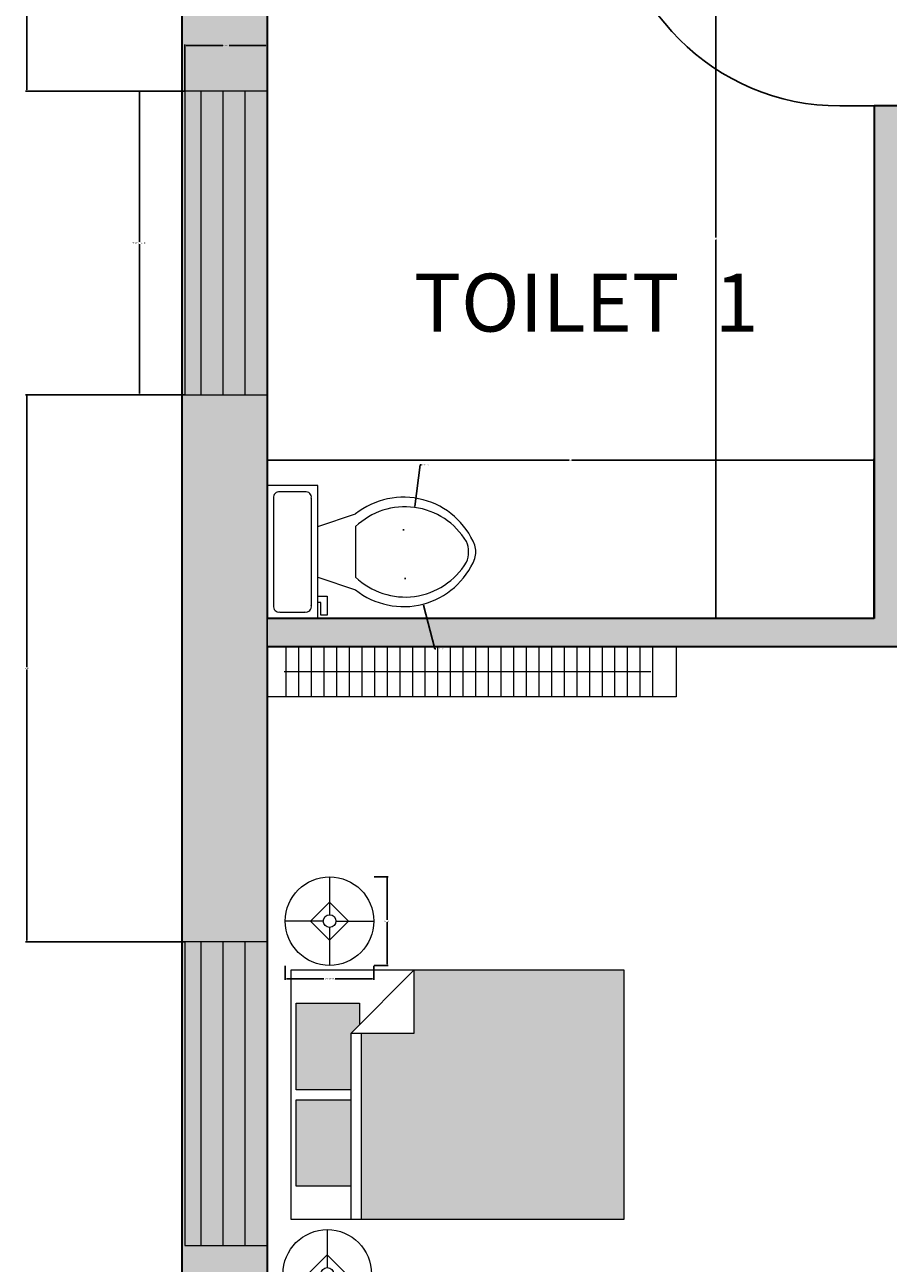
# Model space of a CAD drawing. Units: inches. Extents: x 1434 to 1845, y 1483 to 2014.
# Tile 2 of 11: x 1435 to 1571, y 1633 to 1829. Entities that reach past the tile are written whole.
import ezdxf

# ---------------------------------------------------------------- set-up
doc = ezdxf.new("R2010")
doc.units = ezdxf.units.IN
for name, color, linetype, lineweight in [('A-ANNO-DIMS', 2, 'Continuous', 18), ('A-AREA-IDEN', 7, 'Continuous', 25), ('A-DOOR', 3, 'Continuous', 25), ('A-FLOR-FIXT', 8, 'Continuous', 18), ('A-FLOR-FIXT-PATT', 8, 'Continuous', 13), ('A-FURN', 9, 'Continuous', 18), ('A-FURN-PATT', 9, 'Continuous', 13), ('A-GLAZ', 4, 'Continuous', 18), ('A-GLAZ-PATT', 9, 'Continuous', 13), ('A-WALL', 7, 'Continuous', 35), ('A-WALL-PATT', 8, 'Continuous', 13), ('E-LITE', 2, 'Continuous', 18)]:
    doc.layers.add(name, color=color, linetype=linetype, lineweight=lineweight)
doc.styles.get("Standard").update_dxf_attribs({"font": 'arial.ttf'})
doc.dimstyles.get("Standard").update_dxf_attribs({"dimtxt": 0.18, "dimasz": 0.18, "dimexe": 0.18, "dimexo": 0.0625, "dimgap": 0.09, "dimtad": 0, "dimtih": 1, "dimtoh": 1, "dimdec": 4, "dimzin": 0, "dimdsep": 46, "dimtxsty": 'Standard', "dimcen": 0.09, "dimadec": 0, "dimazin": 0, "dimtfac": 1, "dimtdec": 4, "dimtofl": 0, "dimtmove": 0, "dimatfit": 3, "dimfxl": 1, "dimtolj": 1, "dimtzin": 0, "dimarcsym": 0})

# ---------------------------------------------------------------- blocks, each defined once
blk = doc.blocks.new('*U2')
for p, q in [((0, 0), (0, -6)), ((-40, 0), (-40, -6))]:
    blk.add_line(p, q)
blk.add_lwpolyline([(0, 0), (0, 40), (-1.75, 40), (-1.75, 0)], close=True)
blk.add_arc((0, 0), 40, 90, 180)
blk = doc.blocks.new('Bed - Queen')
for p, q in [((0, -80.00003), (0, 0)), ((0, 0), (59.99999, 0)), ((59.99999, 0), (59.99999, -80.00003)), ((7.99999, -1.2), (28.79998, -1.2)), ((7.99999, -14.4), (7.99999, -1.2)), ((28.79998, -1.2), (28.79998, -14.4)), ((31.19999, -1.2), (51.99999, -1.2)), ((31.19999, -14.4), (31.19999, -1.2)), ((51.99999, -1.2), (51.99999, -16.4)), ((0, -14.4), (44.8, -14.4)), ((59.99999, -29.6), (44.8, -14.4)), ((44.8, -14.4), (44.8, -29.6)), ((44.8, -16.8), (0, -16.8)), ((51.99999, -16.4), (46.79936, -16.4)), ((44.8, -29.6), (59.99999, -29.6)), ((59.99999, -80.00003), (0, -80.00003))]:
    blk.add_line(p, q)
blk = doc.blocks.new('Lamp - Table')
for p, q in [((0, 7), (0, 1)), ((0, 3), (-3, 0)), ((3, 0), (0, 3)), ((-1, 0), (-7, 0)), ((-3, 0), (0, -3)), ((0, -3), (3, 0)), ((1, 0), (7, 0)), ((0, -1), (0, -7))]:
    blk.add_line(p, q)
for radius in [7, 1]:
    blk.add_circle((0, 0), radius)
blk = doc.blocks.new('Toilet - top')
for p, q in [((9.5, -6), (9.5, -2)), ((-10, -8.5), (-8, -8.5)), ((-10, -9.5), (-10, -8.5)), ((-7, -9.5), (-10, -9.5)), ((-8, -8.5), (-8, -8)), ((-7, -8), (-7, -9.5)), ((-4, -8), (-6, -14)), ((4, -8), (6, -14)), ((4, -14), (-4, -14))]:
    blk.add_line(p, q)
blk.add_lwpolyline([(10.5, -8), (10.5, 0), (-10.5, 0), (-10.5, -8)], close=True)
for points in [[(8.5, -1), (-8.5, -1)], [(-9.5, -2), (-9.5, -6)], [(-8.5, -7), (8.5, -7)]]:
    blk.add_lwpolyline(points)
for centre, radius, start, end in [((-8.62, -1.88), 0.884, 81.8699, 188.1301), ((8.62, -1.88), 0.884, 351.8699, 98.1301), ((-8.62, -6.12), 0.884, 171.8699, 278.1301), ((8.62, -6.12), 0.884, 261.8699, 8.1301), ((3.52, -21.58), 12.17, 141.4691, 247.9714), ((4.2, -21.82), 11.33, 136.3677, 238.9468), ((-3.52, -21.58), 12.17, 292.0284, 38.5307), ((-4.2, -21.82), 11.33, 301.053, 43.6321), ((0, -27.88), 4, 245.7318, 294.2682), ((0, -29), 4, 254.8605, 285.1395)]:
    blk.add_arc(centre, radius, start, end)
blk = doc.blocks.new('WIN-48IN-13IN')
for p, q in [((13, 48), (0, 48)), ((0, 48), (0, 12)), ((2.5, 48), (2.5, 0)), ((6, 48), (6, 0)), ((9.5, 48), (9.5, 0)), ((0, 12), (0, 0)), ((0, 0), (13, 0))]:
    blk.add_line(p, q)
blk.add_lwpolyline([(13, 48), (13, 0)], close=True)
blk = doc.blocks.new('*D24')
at = {"layer": 'A-ANNO-DIMS', "color": 0, "lineweight": -2, "transparency": 16777216}
for p, q in [((1475.85, 1679.92), (1475.85, 1677.71)), ((1489.85, 1679.92), (1489.85, 1677.71)), ((1476.03, 1677.89), (1481.95, 1677.89)), ((1489.67, 1677.89), (1483.75, 1677.89))]:
    blk.add_line(p, q, dxfattribs=at)
at = {"layer": 'A-ANNO-DIMS', "color": 0, "transparency": 16777216}
for points in [[(1476.03, 1677.92), (1476.03, 1677.86), (1475.85, 1677.89)], [(1489.67, 1677.92), (1489.67, 1677.86), (1489.85, 1677.89)]]:
    blk.add_solid(points, dxfattribs=at)
at = {"layer": 'Defpoints', "color": 0, "transparency": 16777216}
for p in [(1475.85, 1679.99), (1489.85, 1679.99), (1489.85, 1677.89)]:
    blk.add_point(p, dxfattribs=at)
at = {"layer": 'A-ANNO-DIMS', "color": 0, "transparency": 16777216, "insert": (1482.85, 1677.89), "char_height": 0.18, "attachment_point": 5}
blk.add_mtext('\\A1;LAMP 14 TYP.', dxfattribs=at)
blk = doc.blocks.new('*D25')
at = {"layer": 'A-ANNO-DIMS', "color": 0, "lineweight": -2, "transparency": 16777216}
for p, q in [((1489.91, 1693.99), (1492.13, 1693.99)), ((1491.95, 1693.81), (1491.95, 1687.17)), ((1491.95, 1680.17), (1491.95, 1686.81)), ((1489.91, 1679.99), (1492.13, 1679.99))]:
    blk.add_line(p, q, dxfattribs=at)
at = {"layer": 'A-ANNO-DIMS', "color": 0, "transparency": 16777216}
for points in [[(1491.92, 1693.81), (1491.98, 1693.81), (1491.95, 1693.99)], [(1491.92, 1680.17), (1491.98, 1680.17), (1491.95, 1679.99)]]:
    blk.add_solid(points, dxfattribs=at)
at = {"layer": 'Defpoints', "color": 0, "transparency": 16777216}
for p in [(1489.85, 1693.99), (1491.95, 1693.99), (1489.85, 1679.99)]:
    blk.add_point(p, dxfattribs=at)
at = {"layer": 'A-ANNO-DIMS', "color": 0, "transparency": 16777216, "insert": (1491.95, 1686.99), "char_height": 0.18, "attachment_point": 5}
blk.add_mtext('\\A1;14 TYP.', dxfattribs=at)
blk = doc.blocks.new('*D26')
at = {"layer": 'A-ANNO-DIMS', "color": 0, "lineweight": -2, "transparency": 16777216}
for p, q in [((1459.91, 1818.2), (1452.59, 1818.2)), ((1452.77, 1818.02), (1452.77, 1794.38)), ((1452.77, 1770.38), (1452.77, 1794.01)), ((1459.91, 1770.2), (1452.59, 1770.2))]:
    blk.add_line(p, q, dxfattribs=at)
at = {"layer": 'A-ANNO-DIMS', "color": 0, "transparency": 16777216}
for points in [[(1452.74, 1818.02), (1452.8, 1818.02), (1452.77, 1818.2)], [(1452.74, 1770.38), (1452.8, 1770.38), (1452.77, 1770.2)]]:
    blk.add_solid(points, dxfattribs=at)
at = {"layer": 'Defpoints', "color": 0, "transparency": 16777216}
for p in [(1452.77, 1818.2), (1459.97, 1818.2), (1459.97, 1770.2)]:
    blk.add_point(p, dxfattribs=at)
at = {"layer": 'A-ANNO-DIMS', "color": 0, "transparency": 16777216, "insert": (1452.77, 1794.2), "char_height": 0.18, "attachment_point": 5}
blk.add_mtext('\\A1;WINDOW A 48 TYP.', dxfattribs=at)
blk = doc.blocks.new('*D27')
at = {"layer": 'A-ANNO-DIMS', "color": 0, "lineweight": -2, "transparency": 16777216}
for p, q in [((1459.97, 1818.26), (1459.97, 1825.58)), ((1460.15, 1825.4), (1465.95, 1825.4)), ((1472.79, 1825.4), (1466.99, 1825.4)), ((1472.97, 1818.26), (1472.97, 1825.58))]:
    blk.add_line(p, q, dxfattribs=at)
at = {"layer": 'A-ANNO-DIMS', "color": 0, "transparency": 16777216}
for points in [[(1460.15, 1825.43), (1460.15, 1825.37), (1459.97, 1825.4)], [(1472.79, 1825.43), (1472.79, 1825.37), (1472.97, 1825.4)]]:
    blk.add_solid(points, dxfattribs=at)
at = {"layer": 'Defpoints', "color": 0, "transparency": 16777216}
for p in [(1472.97, 1825.4), (1459.97, 1818.2), (1472.97, 1818.2)]:
    blk.add_point(p, dxfattribs=at)
at = {"layer": 'A-ANNO-DIMS', "color": 0, "transparency": 16777216, "insert": (1466.47, 1825.4), "char_height": 0.18, "attachment_point": 5}
blk.add_mtext('\\A1;13 TYP.', dxfattribs=at)
blk = doc.blocks.new('*D56')
at = {"layer": 'A-ANNO-DIMS', "color": 0, "lineweight": -2, "transparency": 16777216}
for p, q in [((1472.97, 1974.79), (1472.97, 1483.15)), ((1612.47, 1974.79), (1612.47, 1483.15)), ((1473.15, 1483.33), (1542.34, 1483.33)), ((1612.29, 1483.33), (1543.11, 1483.33))]:
    blk.add_line(p, q, dxfattribs=at)
at = {"layer": 'A-ANNO-DIMS', "color": 0, "transparency": 16777216}
for points in [[(1473.15, 1483.36), (1473.15, 1483.3), (1472.97, 1483.33)], [(1612.29, 1483.36), (1612.29, 1483.3), (1612.47, 1483.33)]]:
    blk.add_solid(points, dxfattribs=at)
at = {"layer": 'Defpoints', "color": 0, "transparency": 16777216}
for p in [(1472.97, 1974.86), (1612.47, 1974.86), (1612.47, 1483.33)]:
    blk.add_point(p, dxfattribs=at)
at = {"layer": 'A-ANNO-DIMS', "color": 0, "transparency": 16777216, "insert": (1542.72, 1483.33), "char_height": 0.18, "attachment_point": 5}
blk.add_mtext('\\A1;139.5', dxfattribs=at)
blk = doc.blocks.new('*D61')
at = {"layer": 'A-ANNO-DIMS', "color": 0, "lineweight": -2, "transparency": 16777216}
for p, q in [((1472.97, 1734.92), (1472.97, 1760.06)), ((1473.15, 1759.88), (1520.76, 1759.88)), ((1568.79, 1759.88), (1521.19, 1759.88)), ((1568.97, 1734.92), (1568.97, 1760.06))]:
    blk.add_line(p, q, dxfattribs=at)
at = {"layer": 'A-ANNO-DIMS', "color": 0, "transparency": 16777216}
for points in [[(1473.15, 1759.91), (1473.15, 1759.85), (1472.97, 1759.88)], [(1568.79, 1759.91), (1568.79, 1759.85), (1568.97, 1759.88)]]:
    blk.add_solid(points, dxfattribs=at)
at = {"layer": 'Defpoints', "color": 0, "transparency": 16777216}
for p in [(1568.97, 1759.88), (1472.97, 1734.86), (1568.97, 1734.86)]:
    blk.add_point(p, dxfattribs=at)
at = {"layer": 'A-ANNO-DIMS', "color": 0, "transparency": 16777216, "insert": (1520.97, 1759.88), "char_height": 0.18, "attachment_point": 5}
blk.add_mtext('\\A1;96', dxfattribs=at)
blk = doc.blocks.new('*D63')
at = {"layer": 'A-ANNO-DIMS', "color": 0, "lineweight": -2, "transparency": 16777216}
for p, q in [((1568.91, 1854.86), (1543.77, 1854.86)), ((1543.95, 1854.68), (1543.95, 1795.04)), ((1543.95, 1735.04), (1543.95, 1794.67)), ((1568.91, 1734.86), (1543.77, 1734.86))]:
    blk.add_line(p, q, dxfattribs=at)
at = {"layer": 'A-ANNO-DIMS', "color": 0, "transparency": 16777216}
for points in [[(1543.92, 1854.68), (1543.98, 1854.68), (1543.95, 1854.86)], [(1543.92, 1735.04), (1543.98, 1735.04), (1543.95, 1734.86)]]:
    blk.add_solid(points, dxfattribs=at)
at = {"layer": 'Defpoints', "color": 0, "transparency": 16777216}
for p in [(1543.95, 1854.86), (1568.97, 1854.86), (1568.97, 1734.86)]:
    blk.add_point(p, dxfattribs=at)
at = {"layer": 'A-ANNO-DIMS', "color": 0, "transparency": 16777216, "insert": (1543.95, 1794.86), "char_height": 0.18, "attachment_point": 5}
blk.add_mtext('\\A1;120', dxfattribs=at)
blk = doc.blocks.new('*D77')
at = {"layer": 'A-ANNO-DIMS', "color": 0, "lineweight": -2, "transparency": 16777216}
for p, q in [((1459.91, 1899.94), (1434.77, 1899.94)), ((1434.95, 1899.76), (1434.95, 1859.25)), ((1434.95, 1818.38), (1434.95, 1858.88)), ((1459.91, 1818.2), (1434.77, 1818.2))]:
    blk.add_line(p, q, dxfattribs=at)
at = {"layer": 'A-ANNO-DIMS', "color": 0, "transparency": 16777216}
for points in [[(1434.92, 1899.76), (1434.98, 1899.76), (1434.95, 1899.94)], [(1434.92, 1818.38), (1434.98, 1818.38), (1434.95, 1818.2)]]:
    blk.add_solid(points, dxfattribs=at)
at = {"layer": 'Defpoints', "color": 0, "transparency": 16777216}
for p in [(1434.95, 1899.94), (1459.97, 1899.94), (1459.97, 1818.2)]:
    blk.add_point(p, dxfattribs=at)
at = {"layer": 'A-ANNO-DIMS', "color": 0, "transparency": 16777216, "insert": (1434.95, 1859.07), "char_height": 0.18, "attachment_point": 5}
blk.add_mtext('\\A1;81.74', dxfattribs=at)
blk = doc.blocks.new('*D78')
at = {"layer": 'A-ANNO-DIMS', "color": 0, "lineweight": -2, "transparency": 16777216}
for p, q in [((1459.91, 1770.2), (1434.77, 1770.2)), ((1434.95, 1770.02), (1434.95, 1727.14)), ((1434.95, 1683.91), (1434.95, 1726.78)), ((1459.91, 1683.73), (1434.77, 1683.73))]:
    blk.add_line(p, q, dxfattribs=at)
at = {"layer": 'A-ANNO-DIMS', "color": 0, "transparency": 16777216}
for points in [[(1434.92, 1770.02), (1434.98, 1770.02), (1434.95, 1770.2)], [(1434.92, 1683.91), (1434.98, 1683.91), (1434.95, 1683.73)]]:
    blk.add_solid(points, dxfattribs=at)
at = {"layer": 'Defpoints', "color": 0, "transparency": 16777216}
for p in [(1434.95, 1770.2), (1459.97, 1770.2), (1459.97, 1683.73)]:
    blk.add_point(p, dxfattribs=at)
at = {"layer": 'A-ANNO-DIMS', "color": 0, "transparency": 16777216, "insert": (1434.95, 1726.96), "char_height": 0.18, "attachment_point": 5}
blk.add_mtext('\\A1;86.47', dxfattribs=at)
blk = doc.blocks.new('*D96')
at = {"layer": 'A-ANNO-DIMS', "color": 0, "lineweight": -2, "transparency": 16777216}
for p, q in [((1494.46, 1748.87), (1494.64, 1748.87)), ((1494.55, 1748.78), (1494.55, 1748.96)), ((1499.5, 1730.04), (1497.69, 1736.93)), ((1499.68, 1730.04), (1499.5, 1730.04))]:
    blk.add_line(p, q, dxfattribs=at)
at = {"layer": 'A-ANNO-DIMS', "color": 0, "transparency": 16777216}
blk.add_solid([(1497.72, 1736.94), (1497.66, 1736.92), (1497.65, 1737.11)], dxfattribs=at)
at = {"layer": 'Defpoints', "color": 0, "transparency": 16777216}
for p in [(1494.55, 1748.87), (1497.65, 1737.11)]:
    blk.add_point(p, dxfattribs=at)
at = {"layer": 'A-ANNO-DIMS', "color": 0, "transparency": 16777216, "insert": (1500.36, 1730.04), "char_height": 0.18, "attachment_point": 5}
blk.add_mtext('\\A1;4X R12.17', dxfattribs=at)
blk = doc.blocks.new('*D97')
at = {"layer": 'A-ANNO-DIMS', "color": 0, "lineweight": -2, "transparency": 16777216}
for p, q in [((1497.21, 1759.12), (1496.32, 1752.56)), ((1497.39, 1759.12), (1497.21, 1759.12)), ((1494.7, 1741.16), (1494.88, 1741.16)), ((1494.79, 1741.07), (1494.79, 1741.25))]:
    blk.add_line(p, q, dxfattribs=at)
at = {"layer": 'A-ANNO-DIMS', "color": 0, "transparency": 16777216}
blk.add_solid([(1496.3, 1752.57), (1496.35, 1752.56), (1496.3, 1752.38)], dxfattribs=at)
at = {"layer": 'Defpoints', "color": 0, "transparency": 16777216}
for p in [(1496.3, 1752.38), (1494.79, 1741.16)]:
    blk.add_point(p, dxfattribs=at)
at = {"layer": 'A-ANNO-DIMS', "color": 0, "transparency": 16777216, "insert": (1498.06, 1759.12), "char_height": 0.18, "attachment_point": 5}
blk.add_mtext('\\A1;4X R11.33', dxfattribs=at)

msp = doc.modelspace()

# ---------------------------------------------------------------- hatches: boundary and pattern name
at = {"layer": 'A-FLOR-FIXT-PATT'}
h = msp.add_hatch(dxfattribs=at)
h.set_pattern_fill('ANSI31', color=256, scale=0.629921, angle=45, style=0)
h.paths.add_polyline_path([(1474.6905, 1722.463), (1534.6905, 1722.463), (1534.6905, 1730.3553), (1474.6905, 1730.3553)])
at = {"layer": 'A-FURN-PATT'}
h = msp.add_hatch(color=256, dxfattribs=at)
h.dxf.hatch_style = 1
h.paths.add_polyline_path([(1528.2614, 1944.8381), (1495.0961, 1944.8381), (1495.0961, 1934.8359), (1486.6731, 1934.8359), (1486.6731, 1905.3556), (1528.2614, 1905.3556)])
h.paths.add_polyline_path([(1796.7541, 1950.9116), (1755.1658, 1950.9116), (1755.1658, 1911.4291), (1788.3311, 1911.4291), (1788.3311, 1921.4313), (1796.7541, 1921.4313)])
h.paths.add_polyline_path([(1529.423, 1679.282), (1496.2577, 1679.282), (1496.2577, 1669.2798), (1487.8347, 1669.2798), (1487.8347, 1639.7996), (1529.423, 1639.7996)])
h.paths.add_polyline_path([(1486.2554, 1669.2798), (1487.5715, 1670.5959), (1487.5715, 1674.0177), (1477.5693, 1674.0177), (1477.5693, 1660.3304), (1486.2554, 1660.3304)])
h.paths.add_polyline_path([(1486.2554, 1658.7511), (1477.5693, 1658.7511), (1477.5693, 1645.0639), (1486.2554, 1645.0639)])
h.paths.add_polyline_path([(1807.0195, 1930.3807), (1798.3334, 1930.3807), (1798.3334, 1921.4313), (1797.0173, 1920.1152), (1797.0173, 1916.6934), (1807.0195, 1916.6934)])
h.paths.add_polyline_path([(1807.0195, 1945.6472), (1798.3334, 1945.6472), (1798.3334, 1931.96), (1807.0195, 1931.96)])
h.paths.add_polyline_path([(1485.0938, 1934.8359), (1486.4099, 1936.152), (1486.4099, 1939.5738), (1476.4077, 1939.5738), (1476.4077, 1925.8865), (1485.0938, 1925.8865)])
h.paths.add_polyline_path([(1485.0938, 1924.3072), (1476.4077, 1924.3072), (1476.4077, 1910.62), (1485.0938, 1910.62)])
at = {"layer": 'A-GLAZ-PATT'}
h = msp.add_hatch(color=256, dxfattribs=at)
h.dxf.hatch_style = 1
h.set_gradient(color1=(0, 0, 255), color2=(255, 255, 0), name='INVHEMISPHERICAL')
h.paths.add_polyline_path([(1469.4742, 1818.1951), (1465.9742, 1818.1951), (1465.9742, 1770.1951), (1469.4742, 1770.1951)])
h.paths.add_polyline_path([(1472.9742, 1818.1951), (1469.4742, 1818.1951), (1469.4742, 1770.1951), (1472.9742, 1770.1951)])
h.paths.add_polyline_path([(1462.4742, 1818.1951), (1459.9742, 1818.1951), (1459.9742, 1782.1951), (1459.9742, 1770.1951), (1462.4742, 1770.1951)])
h.paths.add_polyline_path([(1465.9742, 1818.1951), (1462.4742, 1818.1951), (1462.4742, 1770.1951), (1465.9742, 1770.1951)])
h = msp.add_hatch(color=256, dxfattribs=at)
h.dxf.hatch_style = 1
h.set_gradient(color1=(0, 0, 255), color2=(255, 255, 0))
h.paths.add_polyline_path([(1472.9742, 1683.7299), (1469.4742, 1683.7299), (1469.4742, 1635.7299), (1472.9742, 1635.7299)])
h.paths.add_polyline_path([(1469.4742, 1683.7299), (1465.9742, 1683.7299), (1465.9742, 1635.7299), (1469.4742, 1635.7299)])
h.paths.add_polyline_path([(1465.9742, 1683.7299), (1462.4742, 1683.7299), (1462.4742, 1635.7299), (1465.9742, 1635.7299)])
h.paths.add_polyline_path([(1462.4742, 1683.7299), (1459.9742, 1683.7299), (1459.9742, 1647.7299), (1459.9742, 1635.7299), (1462.4742, 1635.7299)])
at = {"layer": 'A-WALL-PATT'}
h = msp.add_hatch(color=256, dxfattribs=at)
h.dxf.hatch_style = 1
h.paths.add_polyline_path([(1472.9742, 1730.3553), (1577.9742, 1730.3553), (1577.9742, 1734.8553), (1573.4742, 1734.8553), (1573.4742, 1815.8553), (1568.9742, 1815.8553), (1568.9742, 1734.8553), (1472.9742, 1734.8553), (1472.9742, 1770.1951), (1459.9742, 1770.1951), (1459.9742, 1782.1951), (1459.9742, 1818.1951), (1472.9742, 1818.1951), (1472.9742, 1854.8553), (1568.9742, 1854.8553), (1568.9742, 1851.8553), (1573.4742, 1851.8553), (1573.4742, 1854.8553), (1573.4742, 1859.3553), (1472.9742, 1859.3553), (1472.9742, 1899.9369), (1459.9742, 1899.9369), (1459.9742, 1911.9369), (1459.9742, 1947.9369), (1472.9742, 1947.9369), (1472.9742, 1974.8553), (1513.9785, 1974.8553), (1513.9785, 1987.8553), (1561.9785, 1987.8553), (1561.9785, 1974.8553), (1612.4742, 1974.8553), (1612.4742, 1859.3553), (1609.4742, 1859.3553), (1609.4742, 1854.8553), (1616.9742, 1854.8553), (1616.9742, 1910.3553), (1625.153, 1910.3553), (1625.153, 1914.8553), (1616.9742, 1914.8553), (1616.9742, 1988.3553), (1459.4742, 1988.3553), (1459.4742, 1508.3553), (1630.4742, 1508.3553), (1630.4742, 1517.3553), (1472.9742, 1517.3553), (1472.9742, 1586.3553), (1616.9742, 1586.3553), (1616.9742, 1583.3553), (1621.4742, 1583.3553), (1621.4742, 1586.3553), (1621.4742, 1734.8553), (1616.9742, 1734.8553), (1613.9742, 1734.8553), (1613.9742, 1730.3553), (1616.9742, 1730.3553), (1616.9742, 1590.8553), (1472.9742, 1590.8553), (1472.9742, 1635.7299), (1459.9742, 1635.7299), (1459.9742, 1647.7299), (1459.9742, 1683.7299), (1472.9742, 1683.7299)])
h.paths.add_polyline_path([(1819.4742, 1773.1667), (1810.4742, 1773.1667), (1810.4742, 1734.8553), (1714.4742, 1734.8553), (1714.4742, 1815.8553), (1709.9742, 1815.8553), (1709.9742, 1730.3553), (1745.9742, 1730.3553), (1745.9742, 1675.0848), (1753.4742, 1675.0848), (1753.4742, 1679.5848), (1750.4742, 1679.5848), (1750.4742, 1730.3553), (1810.4742, 1730.3553), (1810.4742, 1679.5848), (1792.4742, 1679.5848), (1792.4742, 1675.0848), (1810.4742, 1675.0848), (1810.4742, 1517.3553), (1775.1129, 1517.3553), (1775.1129, 1508.3553), (1819.4742, 1508.3553)])
h.paths.add_polyline_path([(1739.1129, 1517.3553), (1694.9742, 1517.3553), (1694.9742, 1730.3553), (1690.4742, 1730.3553), (1690.4742, 1517.3553), (1678.4742, 1517.3553), (1675.4742, 1517.3553), (1672.8212, 1517.3553), (1672.8212, 1508.3553), (1678.4742, 1508.3553), (1739.1129, 1508.3553)])
h.paths.add_polyline_path([(1735.6549, 1987.8553), (1783.6549, 1987.8553), (1783.6549, 1974.8553), (1810.4742, 1974.8553), (1810.4742, 1859.3553), (1709.9742, 1859.3553), (1709.9742, 1854.8553), (1709.9742, 1851.8553), (1714.4742, 1851.8553), (1714.4742, 1854.8553), (1810.4742, 1854.8553), (1810.4742, 1809.1667), (1819.4742, 1809.1667), (1819.4742, 1988.3553), (1666.4742, 1988.3553), (1666.4742, 1914.8553), (1661.1087, 1914.8553), (1661.1087, 1910.3553), (1666.4742, 1910.3553), (1666.4742, 1854.8553), (1673.9742, 1854.8553), (1673.9742, 1859.3553), (1670.9742, 1859.3553), (1670.9742, 1974.8553), (1735.6549, 1974.8553)])

# ---------------------------------------------------------------- linework, layer by layer
at = {"layer": 'A-FLOR-FIXT'}
for p, q in [((1472.9742, 1730.3553), (1537.6905, 1730.3553)), ((1472.9742, 1722.463), (1472.9742, 1730.3553)), ((1537.6905, 1730.3553), (1537.6905, 1722.463)), ((1533.6905, 1726.4092), (1475.6905, 1726.4092)), ((1537.6905, 1722.463), (1472.9742, 1722.463))]:
    msp.add_line(p, q, dxfattribs=at)
at = {"layer": 'A-WALL'}
for p, q in [((1472.9742, 1854.8553), (1472.9742, 1734.8553)), ((1573.4742, 1815.8553), (1568.9742, 1815.8553)), ((1568.9742, 1815.8553), (1568.9742, 1734.8553)), ((1568.9742, 1734.8553), (1472.9742, 1734.8553)), ((1577.9742, 1730.3553), (1472.9742, 1730.3553)), ((1472.9742, 1730.3553), (1472.9742, 1590.8553))]:
    msp.add_line(p, q, dxfattribs=at)
msp.add_lwpolyline([(1678.4742, 1508.3553), (1819.4742, 1508.3553), (1819.4742, 1988.3553), (1459.4742, 1988.3553), (1459.4742, 1508.3553), (1630.4742, 1508.3553)], dxfattribs=at)

# ---------------------------------------------------------------- block references
at = {"layer": 'A-DOOR', "xscale": 0.8979587755198419, "yscale": 0.8979587755198419, "zscale": 0.8979587755198419, "rotation": 90}
msp.add_blockref('*U2', (1563.5864, 1851.7737), dxfattribs=at)
at = {"layer": 'A-FLOR-FIXT', "rotation": 90}
msp.add_blockref('Toilet - top', (1472.9742, 1745.3553), dxfattribs=at)
at = {"layer": 'A-FURN', "xscale": 0.6580416786709006, "yscale": 0.6580416786709006, "zscale": 0.6580416786709006, "rotation": 90}
msp.add_blockref('Bed - Queen', (1476.7796, 1639.7996), dxfattribs=at)
at = {"layer": 'A-GLAZ'}
for p in [(1459.9742, 1770.1951), (1459.9742, 1635.7299)]:
    msp.add_blockref('WIN-48IN-13IN', p, dxfattribs=at)
at = {"layer": 'E-LITE'}
for p in [(1482.852, 1686.9872), (1482.4912, 1631.214)]:
    msp.add_blockref('Lamp - Table', p, dxfattribs=at)

# ---------------------------------------------------------------- texts
at = {"layer": 'A-AREA-IDEN'}
msp.add_text('TOILET  1 ', height=9.14668, dxfattribs=at).set_placement((1496.1823, 1780.1915))

# ---------------------------------------------------------------- dimensions: what is measured, and where the dimension line sits
at = {"layer": 'A-ANNO-DIMS'}
for base, p1, p2, override, picture, middle in [((1612.4742, 1483.3303), (1472.9742, 1974.8553), (1612.4742, 1974.8553), {"dimdec": 1, "dimlfac": 1, "dimrnd": 0, "dimzin": 0, "dimdsep": 46, "dimlunit": 2}, '*D56', (1542.7242, 1483.3303)), ((1568.9742, 1759.8803), (1472.9742, 1734.8553), (1568.9742, 1734.8553), {"dimdec": 0, "dimlfac": 1, "dimrnd": 0, "dimzin": 0, "dimdsep": 46, "dimlunit": 2}, '*D61', (1520.9742, 1759.8803))]:
    dim = msp.add_linear_dim(base=base, p1=p1, p2=p2, dimstyle='Standard', override=override, dxfattribs=at)
    dim.commit()
    dim.dimension.update_dxf_attribs({"geometry": picture, "text_midpoint": middle})
for base, p1, p2, override, picture, middle in [((1434.9492, 1899.9369), (1459.9742, 1818.1951), (1459.9742, 1899.9369), {"dimdec": 2, "dimlfac": 1, "dimrnd": 0, "dimzin": 0, "dimdsep": 46, "dimlunit": 2}, '*D77', (1434.9492, 1859.066)), ((1543.9492, 1854.8553), (1568.9742, 1734.8553), (1568.9742, 1854.8553), {"dimdec": 0, "dimlfac": 1, "dimrnd": 0, "dimzin": 0, "dimdsep": 46, "dimlunit": 2}, '*D63', (1543.9492, 1794.8553)), ((1434.9492, 1770.1951), (1459.9742, 1683.7299), (1459.9742, 1770.1951), {"dimdec": 2, "dimlfac": 1, "dimrnd": 0, "dimzin": 0, "dimdsep": 46, "dimlunit": 2}, '*D78', (1434.9492, 1726.9625))]:
    dim = msp.add_linear_dim(base=base, p1=p1, p2=p2, angle=90, dimstyle='Standard', override=override, dxfattribs=at)
    dim.commit()
    dim.dimension.update_dxf_attribs({"geometry": picture, "text_midpoint": middle})
for base, p1, p2, text, picture, middle in [((1472.9742, 1825.3951), (1459.9742, 1818.1951), (1472.9742, 1818.1951), '<> TYP.', '*D27', (1466.4742, 1825.3951)), ((1489.852, 1677.8872), (1475.852, 1679.9872), (1489.852, 1679.9872), 'LAMP <> TYP.', '*D24', (1482.852, 1677.8872))]:
    dim = msp.add_linear_dim(base=base, p1=p1, p2=p2, text=text, dimstyle='Standard', override={"dimdec": 0, "dimlfac": 1, "dimrnd": 0, "dimzin": 0, "dimdsep": 46, "dimlunit": 2}, dxfattribs=at)
    dim.commit()
    dim.dimension.update_dxf_attribs({"geometry": picture, "text_midpoint": middle})
for base, p1, p2, text, picture, middle in [((1452.7742, 1818.1951), (1459.9742, 1770.1951), (1459.9742, 1818.1951), 'WINDOW A <> TYP.', '*D26', (1452.7742, 1794.1951)), ((1491.952, 1693.9872), (1489.852, 1679.9872), (1489.852, 1693.9872), '<> TYP.', '*D25', (1491.952, 1686.9872))]:
    dim = msp.add_linear_dim(base=base, p1=p1, p2=p2, angle=90, text=text, dimstyle='Standard', override={"dimdec": 0, "dimlfac": 1, "dimrnd": 0, "dimzin": 0, "dimdsep": 46, "dimlunit": 2}, dxfattribs=at)
    dim.commit()
    dim.dimension.update_dxf_attribs({"geometry": picture, "text_midpoint": middle})
for center, mpoint, picture, middle in [((1494.7916, 1741.1554), (1496.3009, 1752.3836), '*D97', (1498.0634, 1759.1205)), ((1494.5547, 1748.8749), (1497.6469, 1737.1053), '*D96', (1500.3591, 1730.0435))]:
    dim = msp.add_radius_dim(center=center, mpoint=mpoint, text='4X <>', dimstyle='Standard', override={"dimdec": 2, "dimlfac": 1, "dimrnd": 0, "dimzin": 0, "dimdsep": 46, "dimlunit": 2}, dxfattribs=at)
    dim.commit()
    dim.dimension.update_dxf_attribs({"geometry": picture, "text_midpoint": middle, "dimtype": 164})

doc.saveas('drawing.dxf')
